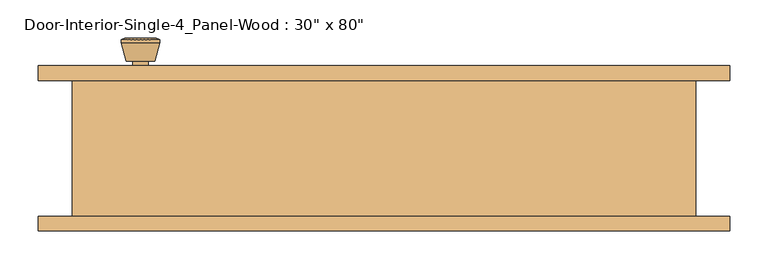
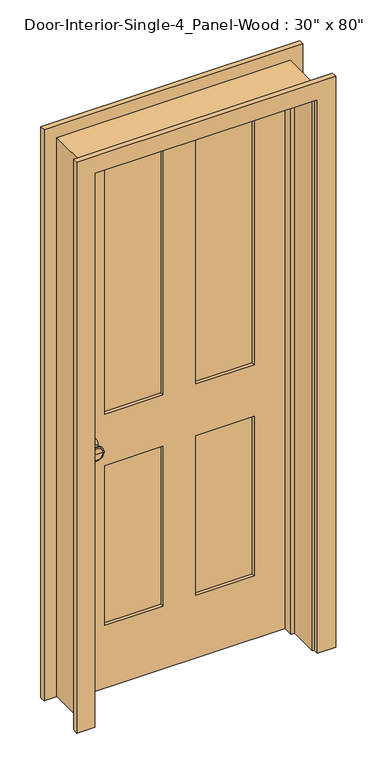
"""IFC4 building model written with IfcOpenShell, lengths in millimetres: door geometry."""

from ifc_helpers import new_model, si_unit, point, frame, frame_2d, origin, place, context, project, spatial, polyline, circle_curve, trimmed, segment, composite_curve, outline, extrude, faceted_brep, source, transform, mapped, element, save
from ifc_brep_helpers import plane_surface, cylinder_surface, revolved_surface, advanced_brep


def door_b97b09b3(model_context):
    return source(origin(), model_context, "Body", "SolidModel", [
        advanced_brep(
        [(-317.5, 44.8, 914.4), (-307.5, 44.8, 914.4), (-327.5, 44.8, 914.4), (-297.0241324, -4.2, 914.4), (-317.5, -4.2, 914.4), (-337.9758676, -4.2, 914.4), (-292.5, -2.3721319, 914.4), (-342.5, -2.3721319, 914.4), (-292.5, 1.0915463, 914.4), (-342.5, 1.0915463, 914.4), (-298.863764, 25.8, 914.4), (-336.136236, 25.8, 914.4), (-307.5, 25.8, 914.4), (-327.5, 25.8, 914.4)],
        [
            (0, 1),
            (1, 2, circle_curve(frame((-317.5, 44.8, 914.4), z_axis=(0.0, 1.0, 0.0), x_axis=(-1.0, 0.0, 0.0)), 10.0)),
            (2, 0),
            (2, 1, circle_curve(frame((-317.5, 44.8, 914.4), z_axis=(0.0, 1.0, 0.0), x_axis=(-1.0, 0.0, 0.0)), 10.0)),
            (3, 4),
            (4, 5),
            (5, 3, circle_curve(frame((-317.5, -4.2, 914.4), z_axis=(0.0, -1.0, 0.0), x_axis=(-1.0, 0.0, 0.0)), 20.4758676)),
            (3, 5, circle_curve(frame((-317.5, -4.2, 914.4), z_axis=(0.0, -1.0, 0.0), x_axis=(-1.0, 0.0, 0.0)), 20.4758676)),
            (6, 3),
            (5, 7),
            (7, 6, circle_curve(frame((-317.5, -2.3721319, 914.4), z_axis=(0.0, -1.0, 0.0), x_axis=(-1.0, 0.0, 0.0)), 25.0)),
            (6, 7, circle_curve(frame((-317.5, -2.3721319, 914.4), z_axis=(0.0, -1.0, 0.0), x_axis=(-1.0, 0.0, 0.0)), 25.0)),
            (8, 6),
            (7, 9),
            (9, 8, circle_curve(frame((-317.5, 1.0915463, 914.4), z_axis=(0.0, -1.0, 0.0), x_axis=(-1.0, 0.0, 0.0)), 25.0)),
            (8, 9, circle_curve(frame((-317.5, 1.0915463, 914.4), z_axis=(0.0, -1.0, 0.0), x_axis=(-1.0, 0.0, 0.0)), 25.0)),
            (10, 8),
            (9, 11),
            (11, 10, circle_curve(frame((-317.5, 25.8, 914.4), z_axis=(0.0, -1.0, 0.0), x_axis=(-1.0, 0.0, 0.0)), 18.636236)),
            (10, 11, circle_curve(frame((-317.5, 25.8, 914.4), z_axis=(0.0, -1.0, 0.0), x_axis=(-1.0, 0.0, 0.0)), 18.636236)),
            (12, 10),
            (11, 13),
            (13, 12, circle_curve(frame((-317.5, 25.8, 914.4), z_axis=(0.0, -1.0, 0.0), x_axis=(-1.0, 0.0, 0.0)), 10.0)),
            (12, 13, circle_curve(frame((-317.5, 25.8, 914.4), z_axis=(0.0, -1.0, 0.0), x_axis=(-1.0, 0.0, 0.0)), 10.0)),
            (1, 12),
            (13, 2),
        ],
        [
            plane_surface(frame((-317.5, 44.8, 914.4), z_axis=(0.0, 1.0, 0.0), x_axis=(-1.0, 0.0, 0.0))),
            plane_surface(frame((-317.5, -4.2, 914.4), z_axis=(0.0, -1.0, 0.0), x_axis=(-1.0, 0.0, 0.0))),
            revolved_surface(polyline([(-337.9758676, -4.2, 914.4), (-342.5, -2.3721319, 914.4)]), (-317.5, 44.8, 914.4), (0.0, 1.0, 0.0)),
            cylinder_surface(frame((-317.5, 44.8, 914.4), z_axis=(0.0, 1.0, 0.0), x_axis=(-1.0, 0.0, 0.0)), 25.0),
            revolved_surface(polyline([(-342.5, 1.0915463, 914.4), (-336.136236, 25.8, 914.4)]), (-317.5, 44.8, 914.4), (0.0, 1.0, 0.0)),
            plane_surface(frame((-317.5, 25.8, 914.4), z_axis=(0.0, 1.0, 0.0), x_axis=(-1.0, 0.0, 0.0))),
            cylinder_surface(frame((-317.5, 44.8, 914.4), z_axis=(0.0, 1.0, 0.0), x_axis=(-1.0, 0.0, 0.0)), 10.0),
        ],
        [
            (0, [[1, 2, 3]]),
            (0, [[-3, 4, -1]]),
            (1, [[5, 6, 7]]),
            (1, [[-6, -5, 8]]),
            (2, [[9, -7, 10, 11]]),
            (2, [[-10, -8, -9, 12]]),
            (3, [[13, -11, 14, 15]]),
            (3, [[-14, -12, -13, 16]]),
            (4, [[17, -15, 18, 19]]),
            (4, [[-18, -16, -17, 20]]),
            (5, [[21, -19, 22, 23]]),
            (5, [[-22, -20, -21, 24]]),
            (6, [[25, -23, 26, -2]]),
            (6, [[-26, -24, -25, -4]]),
        ],
    ),
        extrude(outline(composite_curve([segment(trimmed(circle_curve(frame_2d((914.4, -317.5)), 30.0), [point((914.4, -347.5))], [point((914.4, -287.5))], False, "CARTESIAN"), True, "CONTINUOUS"), segment(trimmed(circle_curve(frame_2d((914.4, -317.5)), 30.0), [point((914.4, -287.5))], [point((914.4, -347.5))], False, "CARTESIAN"), True, "CONTINUOUS")], self_intersect=False)), frame((0.0, 44.8, 0.0), z_axis=(0.0, 1.0, 0.0), x_axis=(0.0, 0.0, 1.0)), (0.0, 0.0, 1.0), 6.0),
        advanced_brep(
        [(-317.5, 91.725, 914.4), (-327.5, 91.725, 914.4), (-307.5, 91.725, 914.4), (-297.0241324, 140.725, 914.4), (-337.9758676, 140.725, 914.4), (-317.5, 140.725, 914.4), (-292.5, 138.8971319, 914.4), (-342.5, 138.8971319, 914.4), (-292.5, 135.4334537, 914.4), (-342.5, 135.4334537, 914.4), (-298.863764, 110.725, 914.4), (-336.136236, 110.725, 914.4), (-307.5, 110.725, 914.4), (-327.5, 110.725, 914.4)],
        [
            (0, 1),
            (1, 2, circle_curve(frame((-317.5, 91.725, 914.4), z_axis=(0.0, -1.0, 0.0), x_axis=(-1.0, 0.0, 0.0)), 10.0)),
            (2, 0),
            (2, 1, circle_curve(frame((-317.5, 91.725, 914.4), z_axis=(0.0, -1.0, 0.0), x_axis=(-1.0, 0.0, 0.0)), 10.0)),
            (3, 4, circle_curve(frame((-317.5, 140.725, 914.4), z_axis=(0.0, 1.0, 0.0), x_axis=(-1.0, 0.0, 0.0)), 20.4758676)),
            (4, 5),
            (5, 3),
            (4, 3, circle_curve(frame((-317.5, 140.725, 914.4), z_axis=(0.0, 1.0, 0.0), x_axis=(-1.0, 0.0, 0.0)), 20.4758676)),
            (6, 7, circle_curve(frame((-317.5, 138.8971319, 914.4), z_axis=(0.0, 1.0, 0.0), x_axis=(-1.0, 0.0, 0.0)), 25.0)),
            (7, 4),
            (3, 6),
            (7, 6, circle_curve(frame((-317.5, 138.8971319, 914.4), z_axis=(0.0, 1.0, 0.0), x_axis=(-1.0, 0.0, 0.0)), 25.0)),
            (8, 9, circle_curve(frame((-317.5, 135.4334537, 914.4), z_axis=(0.0, 1.0, 0.0), x_axis=(-1.0, 0.0, 0.0)), 25.0)),
            (9, 7),
            (6, 8),
            (9, 8, circle_curve(frame((-317.5, 135.4334537, 914.4), z_axis=(0.0, 1.0, 0.0), x_axis=(-1.0, 0.0, 0.0)), 25.0)),
            (10, 11, circle_curve(frame((-317.5, 110.725, 914.4), z_axis=(0.0, 1.0, 0.0), x_axis=(-1.0, 0.0, 0.0)), 18.636236)),
            (11, 9),
            (8, 10),
            (11, 10, circle_curve(frame((-317.5, 110.725, 914.4), z_axis=(0.0, 1.0, 0.0), x_axis=(-1.0, 0.0, 0.0)), 18.636236)),
            (12, 13, circle_curve(frame((-317.5, 110.725, 914.4), z_axis=(0.0, 1.0, 0.0), x_axis=(-1.0, 0.0, 0.0)), 10.0)),
            (13, 11),
            (10, 12),
            (13, 12, circle_curve(frame((-317.5, 110.725, 914.4), z_axis=(0.0, 1.0, 0.0), x_axis=(-1.0, 0.0, 0.0)), 10.0)),
            (1, 13),
            (12, 2),
        ],
        [
            plane_surface(frame((-317.5, 91.725, 914.4), z_axis=(0.0, -1.0, 0.0), x_axis=(-1.0, 0.0, 0.0))),
            plane_surface(frame((-317.5, 140.725, 914.4), z_axis=(0.0, 1.0, 0.0), x_axis=(-1.0, 0.0, 0.0))),
            revolved_surface(polyline([(-337.9758676, 140.725, 914.4), (-342.5, 138.8971319, 914.4)]), (-317.5, 91.725, 914.4), (0.0, -1.0, 0.0)),
            cylinder_surface(frame((-317.5, 91.725, 914.4), z_axis=(0.0, -1.0, 0.0), x_axis=(-1.0, 0.0, 0.0)), 25.0),
            revolved_surface(polyline([(-342.5, 135.4334537, 914.4), (-336.136236, 110.725, 914.4)]), (-317.5, 91.725, 914.4), (0.0, -1.0, 0.0)),
            plane_surface(frame((-317.5, 110.725, 914.4), z_axis=(0.0, -1.0, 0.0), x_axis=(-1.0, 0.0, 0.0))),
            cylinder_surface(frame((-317.5, 91.725, 914.4), z_axis=(0.0, -1.0, 0.0), x_axis=(-1.0, 0.0, 0.0)), 10.0),
        ],
        [
            (0, [[1, 2, 3]]),
            (0, [[-3, 4, -1]]),
            (1, [[5, 6, 7]]),
            (1, [[8, -7, -6]]),
            (2, [[9, 10, -5, 11]]),
            (2, [[12, -11, -8, -10]]),
            (3, [[13, 14, -9, 15]]),
            (3, [[16, -15, -12, -14]]),
            (4, [[17, 18, -13, 19]]),
            (4, [[20, -19, -16, -18]]),
            (5, [[21, 22, -17, 23]]),
            (5, [[24, -23, -20, -22]]),
            (6, [[-2, 25, -21, 26]]),
            (6, [[-4, -26, -24, -25]]),
        ],
    ),
        extrude(outline(composite_curve([segment(trimmed(circle_curve(frame_2d((914.4, -317.5)), 30.0), [point((914.4, -347.5))], [point((914.4, -287.5))], False, "CARTESIAN"), True, "CONTINUOUS"), segment(trimmed(circle_curve(frame_2d((914.4, -317.5)), 30.0), [point((914.4, -287.5))], [point((914.4, -347.5))], False, "CARTESIAN"), True, "CONTINUOUS")], self_intersect=False)), frame((0.0, 85.725, 0.0), z_axis=(0.0, 1.0, 0.0), x_axis=(0.0, 0.0, 1.0)), (0.0, 0.0, 1.0), 6.0),
        extrude(outline(polyline([(260.35, 62.4416667), (57.15, 62.4416667), (57.15, 74.0833333), (260.35, 74.0833333), (260.35, 62.4416667)])), frame((0.0, 0.0, 1009.65), z_axis=(0.0, 0.0, 1.0), x_axis=(1.0, 0.0, 0.0)), (0.0, 0.0, 1.0), 903.2875),
        extrude(outline(polyline([(-57.15, 62.4416667), (-260.35, 62.4416667), (-260.35, 74.0833333), (-57.15, 74.0833333), (-57.15, 62.4416667)])), frame((0.0, 0.0, 1009.65), z_axis=(0.0, 0.0, 1.0), x_axis=(1.0, 0.0, 0.0)), (0.0, 0.0, 1.0), 903.2875),
        extrude(outline(polyline([(260.35, 62.4416667), (57.15, 62.4416667), (57.15, 74.0833333), (260.35, 74.0833333), (260.35, 62.4416667)])), frame((0.0, 0.0, 231.775), z_axis=(0.0, 0.0, 1.0), x_axis=(1.0, 0.0, 0.0)), (0.0, 0.0, 1.0), 587.375),
        extrude(outline(polyline([(-57.15, 62.4416667), (-260.35, 62.4416667), (-260.35, 74.0833333), (-57.15, 74.0833333), (-57.15, 62.4416667)])), frame((0.0, 0.0, 231.775), z_axis=(0.0, 0.0, 1.0), x_axis=(1.0, 0.0, 0.0)), (0.0, 0.0, 1.0), 587.375),
        extrude(outline(polyline([(2032.0, -381.0), (0.0, -381.0), (0.0, 381.0), (2032.0, 381.0), (2032.0, -381.0)]), holes=[polyline([(1912.9375, 57.15), (1912.9375, 260.35), (1009.65, 260.35), (1009.65, 57.15), (1912.9375, 57.15)]), polyline([(1009.65, -57.15), (1009.65, -260.35), (1912.9375, -260.35), (1912.9375, -57.15), (1009.65, -57.15)]), polyline([(819.15, 57.15), (819.15, 260.35), (231.775, 260.35), (231.775, 57.15), (819.15, 57.15)]), polyline([(231.775, -57.15), (231.775, -260.35), (819.15, -260.35), (819.15, -57.15), (231.775, -57.15)])]), frame((0.0, 50.8, 0.0), z_axis=(0.0, 1.0, 0.0), x_axis=(0.0, 0.0, 1.0)), (0.0, 0.0, 1.0), 34.925),
        faceted_brep([(406.4, 85.725, 0.0), (406.4, -92.075, 0.0), (381.0, -92.075, 0.0), (381.0, 15.875, 0.0), (368.3, 15.875, 0.0), (368.3, 50.8, 0.0), (381.0, 50.8, 0.0), (381.0, 85.725, 0.0), (406.4, 85.725, 2057.4), (406.4, -92.075, 2057.4), (-406.4, -92.075, 2057.4), (-406.4, -92.075, 0.0), (-381.0, -92.075, 0.0), (-381.0, -92.075, 2032.0), (381.0, -92.075, 2032.0), (381.0, 15.875, 2032.0), (-381.0, 15.875, 2032.0), (-381.0, 15.875, 0.0), (-368.3, 15.875, 0.0), (-368.3, 15.875, 2019.3), (368.3, 15.875, 2019.3), (368.3, 50.8, 2019.3), (-368.3, 50.8, 2019.3), (-368.3, 50.8, 0.0), (-381.0, 50.8, 0.0), (-381.0, 50.8, 2032.0), (381.0, 50.8, 2032.0), (381.0, 85.725, 2032.0), (-381.0, 85.725, 2032.0), (-381.0, 85.725, 0.0), (-406.4, 85.725, 0.0), (-406.4, 85.725, 2057.4)], [[[0, 1, 2, 3, 4, 5, 6, 7]], [[1, 0, 8, 9]], [[2, 1, 9, 10, 11, 12, 13, 14]], [[3, 2, 14, 15]], [[4, 3, 15, 16, 17, 18, 19, 20]], [[5, 4, 20, 21]], [[6, 5, 21, 22, 23, 24, 25, 26]], [[7, 6, 26, 27]], [[0, 7, 27, 28, 29, 30, 31, 8]], [[9, 8, 31, 10]], [[15, 14, 13, 16]], [[21, 20, 19, 22]], [[27, 26, 25, 28]], [[30, 29, 24, 23, 18, 17, 12, 11]], [[10, 31, 30, 11]], [[16, 13, 12, 17]], [[22, 19, 18, 23]], [[28, 25, 24, 29]]]),
        extrude(outline(polyline([(0.0, 387.35), (0.0, 450.85), (2101.85, 450.85), (2101.85, -450.85), (0.0, -450.85), (0.0, -387.35), (2038.35, -387.35), (2038.35, 387.35), (0.0, 387.35)])), frame((0.0, -111.125, 0.0), z_axis=(0.0, 1.0, 0.0), x_axis=(0.0, 0.0, 1.0)), (0.0, 0.0, 1.0), 19.05),
        extrude(outline(polyline([(0.0, 387.35), (0.0, 450.85), (2101.85, 450.85), (2101.85, -450.85), (0.0, -450.85), (0.0, -387.35), (2038.35, -387.35), (2038.35, 387.35), (0.0, 387.35)])), frame((0.0, 85.725, 0.0), z_axis=(0.0, 1.0, 0.0), x_axis=(0.0, 0.0, 1.0)), (0.0, 0.0, 1.0), 19.05),
    ])


if __name__ == "__main__":
    model = new_model("IFC4")
    model_context = context("Model", 3, world=origin())
    ifc_project = project(units=[si_unit("LENGTHUNIT", "METRE", prefix="MILLI")], contexts=[model_context])
    site = spatial("IfcSite", under=ifc_project)
    building = spatial("IfcBuilding", under=site)
    placement = place(None, origin())
    door_shape = door_b97b09b3(model_context)
    element("IfcDoor", 1, ObjectType="Door-Interior-Single-4_Panel-Wood : 30\" x 80\"", at=placement, inside=building, context=model_context, shape_type="MappedRepresentation", body=[
        mapped(door_shape, transform((0.0, 0.0, 0.0), x_axis=(1.0, 0.0, 0.0), y_axis=(0.0, 1.0, 0.0), z_axis=(0.0, 0.0, 1.0))),
    ])
    save(model, "model.ifc")

# Revit data of these elements
# Type "Door-Interior-Single-4_Panel-Wood : 30\" x 80\""
#   Type Mark = "9"
#   Assembly Code = "C1020300"
#   Analytic Construction = "Wooden"
#   Top Rail = 0' - 4 11/16"
#   Thickness = 0' - 1 3/8"
#   Thermal Resistance (R) = 2.5876 (h·ft²·°F)/BTU
#   Swing Angle [instance default] = 90.00°
#   Stiles = 0' - 4 3/4"
#   Rough Width = 2' - 8"
#   Rough Height = 6' - 9"
#   Mullion = 0' - 4 1/2"
#   Lock Rail = 0' - 7 1/2"
#   Height = 6' - 8"
#   Width = 2' - 6"
#   Heat Transfer Coefficient (U) = 0.3865 BTU/(h·ft²·°F)
#   Bottom Rail = 0' - 9 1/8"
#   Trim Material = Cherry
#   Panel Material = Cherry
#   Frame Material = Cherry
#   Door Handle Material = Aluminum
#   Visual Light Transmittance = 0
#   Solar Heat Gain Coefficient = 0
#   Wall Closure = (empty or 0)
#   Function = (empty or 0)
# Element 1 (IfcDoor, "Door-Interior-Single-4_Panel-Wood : 30\" x 80\"")
#   Materials on its faces: "Cherry", "Aluminum"
# Materials
#   "Cherry": class "Wood", colour RGB 226 177 128, transparency 0, Description = "Prunus Serotina", Cost = 0
#   "Aluminum": class "Metal", colour RGB 247 247 247, transparency 0, Description = "Aluminum 6061", Cost = 0
